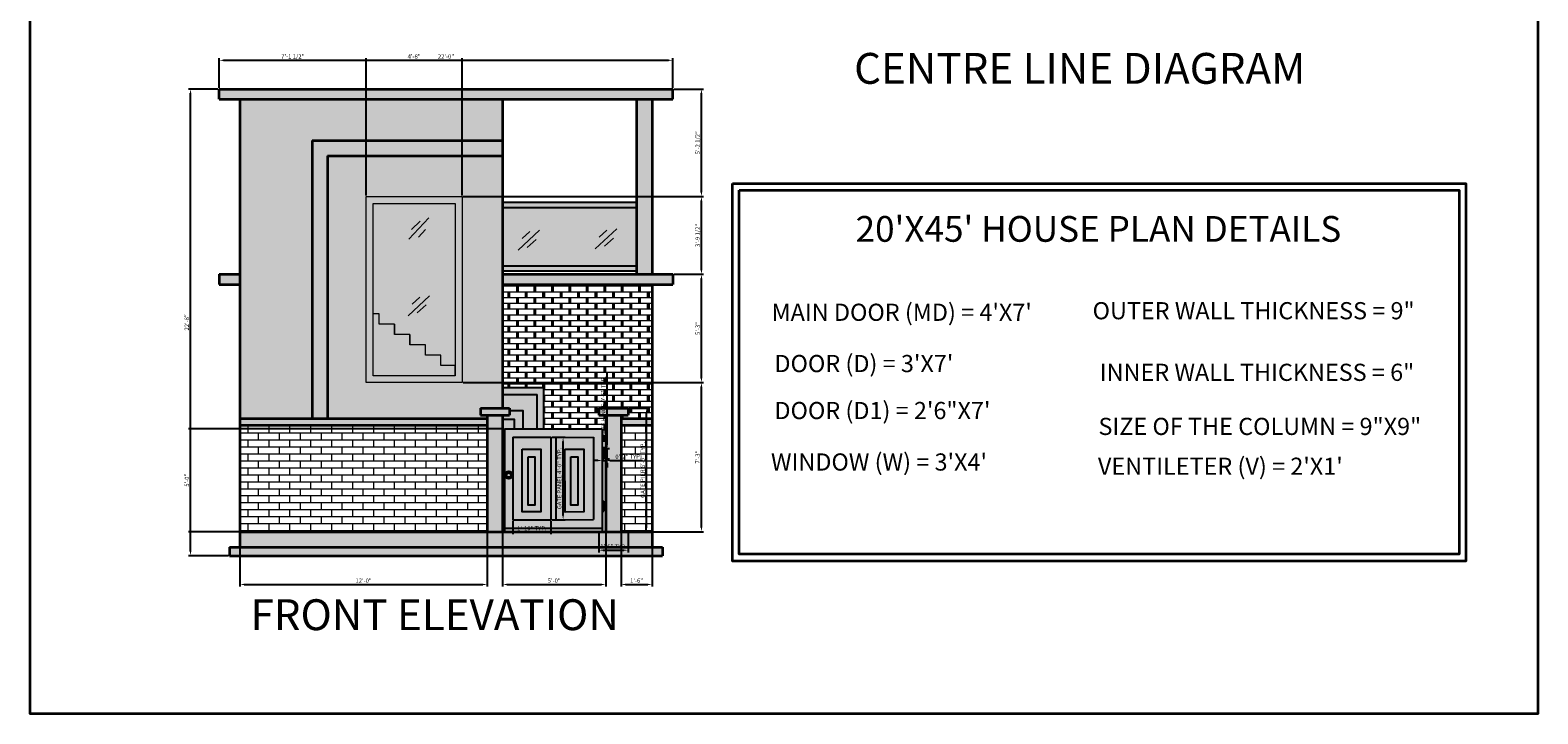
# Model space of a CAD drawing. Units: inches. Extents: x 2150 to 10686, y 1035 to 5077.
# Tile 10 of 12: x 9808 to 10686, y 1035 to 1433. Entities that reach past the tile are written whole.
import ezdxf

# ---------------------------------------------------------------- set-up
doc = ezdxf.new("R2010")
doc.units = ezdxf.units.IN
for name, color, linetype, lineweight in [('A-ANNO-DIMS', 2, 'Continuous', 18), ('A-ANNO-TEXT', 2, 'Continuous', 18), ('A-ANNO-TITL', 3, 'Continuous', 35), ('A-ANNO-TTLB', 7, 'Continuous', 35), ('A-ELEV', 7, 'Continuous', 35), ('A-ELEV-BASE-PATT', 251, 'Continuous', 13), ('A-ELEV-DOOR', 7, 'Continuous', 25), ('A-ELEV-DOOR-PATT', 17, 'Continuous', 13), ('A-ELEV-GLAZ', 7, 'Continuous', 18), ('A-ELEV-MASN-PATT', 32, 'Continuous', 13), ('A-ELEV-METL-PATT', 252, 'Continuous', 13), ('A-ELEV-RAIL', 7, 'Continuous', 25), ('A-ELEV-STRS', 7, 'Continuous', 18)]:
    doc.layers.add(name, color=color, linetype=linetype, lineweight=lineweight)
for name, color, linetype, lineweight, true_color in [('A-ELEV-CONC-PATT', 253, 'Continuous', 13, 0xb2a88f), ('A-ELEV-GLAZ-PATT', 141, 'Continuous', 13, 0xadddf7), ('A-ELEV-PATT', 253, 'Continuous', 13, 0xa5adc8), ('A-ELEV-TRIM-PATT', 85, 'Continuous', 13, 0x58ba48)]:
    doc.layers.add(name, color=color, linetype=linetype, lineweight=lineweight, true_color=true_color)
doc.styles.get("Standard").update_dxf_attribs({"font": 'arial.ttf'})
doc.dimstyles.new('ISO-25', dxfattribs={"dimtxt": 2.5, "dimasz": 2.5, "dimexe": 1.25, "dimexo": 0.625, "dimtad": 1, "dimdec": 0, "dimlunit": 3, "dimtxsty": 'Standard', "dimcen": 2.5, "dimadec": 0, "dimazin": 0, "dimtfac": 1, "dimtdec": 0, "dimtmove": 0, "dimatfit": 3, "dimfxl": 1, "dimarcsym": 0})

# ---------------------------------------------------------------- blocks, each defined once
blk = doc.blocks.new('GLASS-REFLECTION-COMPACT')
for p, q in [((0, 0), (11.74, 12.37)), ((1.57, 5.5), (6.55, 10.47)), ((5.63, 1.12), (9.83, 5.5))]:
    blk.add_line(p, q)
blk = doc.blocks.new('GATE-PIER-CAPPED')
for p, q in [((0, 72), (0, 68)), ((0, 72), (17, 72)), ((17, 72), (17, 68)), ((0, 68), (17, 68)), ((4, 68), (4, 0)), ((13, 68), (13, 0))]:
    blk.add_line(p, q)
blk = doc.blocks.new('GATE-INSET-PANEL-22')
for p, q in [((0, 48), (0, 0)), ((0, 48), (22, 48)), ((22, 48), (22, 0)), ((0, 0), (22, 0))]:
    blk.add_line(p, q)
for points in [[(5.38, 41.12), (16.31, 41.12), (16.31, 4.48), (5.38, 4.48)], [(8.77, 36.65), (12.8, 36.65), (12.8, 8.4), (8.77, 8.4)]]:
    blk.add_lwpolyline(points, close=True)
blk = doc.blocks.new('GATE-HINGE-6IN')
for p, q in [((0, 6), (1, 6)), ((0, 0), (1, 0)), ((1, 6), (1, 0)), ((1, 4), (2, 4)), ((1, 2), (2, 2))]:
    blk.add_line(p, q)
blk = doc.blocks.new('*D68')
at = {"layer": 'A-ANNO-DIMS', "color": 0, "lineweight": -2, "transparency": 16777216}
for p, q in [((10157.13, 1213.1), (10168.56, 1213.1)), ((10167.31, 1143.6), (10167.31, 1210.6)), ((10157.13, 1141.1), (10168.56, 1141.1))]:
    blk.add_line(p, q, dxfattribs=at)
at = {"layer": 'A-ANNO-DIMS', "color": 0, "transparency": 16777216}
for points in [[(10166.89, 1210.6), (10167.72, 1210.6), (10167.31, 1213.1)], [(10166.89, 1143.6), (10167.72, 1143.6), (10167.31, 1141.1)]]:
    blk.add_solid(points, dxfattribs=at)
at = {"layer": 'Defpoints', "color": 0, "transparency": 16777216}
for p in [(10156.51, 1213.1), (10167.31, 1213.1), (10156.51, 1141.1)]:
    blk.add_point(p, dxfattribs=at)
at = {"layer": 'A-ANNO-DIMS', "color": 0, "transparency": 16777216, "insert": (10165.39, 1177.1), "char_height": 2.5, "attachment_point": 5, "rotation": 90}
blk.add_mtext('GATE PIER 6\'-0" TYP.', dxfattribs=at)
blk = doc.blocks.new('*D69')
at = {"layer": 'A-ANNO-DIMS', "color": 0, "lineweight": -2, "transparency": 16777216}
for p, q in [((10139.51, 1140.47), (10139.51, 1129.05)), ((10156.51, 1140.47), (10156.51, 1129.05)), ((10142.01, 1130.3), (10154.01, 1130.3))]:
    blk.add_line(p, q, dxfattribs=at)
at = {"layer": 'A-ANNO-DIMS', "color": 0, "transparency": 16777216}
for points in [[(10142.01, 1130.71), (10142.01, 1129.88), (10139.51, 1130.3)], [(10154.01, 1130.71), (10154.01, 1129.88), (10156.51, 1130.3)]]:
    blk.add_solid(points, dxfattribs=at)
at = {"layer": 'Defpoints', "color": 0, "transparency": 16777216}
for p in [(10139.51, 1141.1), (10156.51, 1141.1), (10156.51, 1130.3)]:
    blk.add_point(p, dxfattribs=at)
at = {"layer": 'A-ANNO-DIMS', "color": 0, "transparency": 16777216, "insert": (10148.01, 1132.2), "char_height": 2.5, "attachment_point": 5}
blk.add_mtext('1\'-5" TYP.', dxfattribs=at)
blk = doc.blocks.new('*D70')
at = {"layer": 'A-ANNO-DIMS', "color": 0, "lineweight": -2, "transparency": 16777216}
for p, q in [((10112.13, 1196.1), (10119.96, 1196.1)), ((10118.71, 1150.6), (10118.71, 1193.6)), ((10112.13, 1148.1), (10119.96, 1148.1))]:
    blk.add_line(p, q, dxfattribs=at)
at = {"layer": 'A-ANNO-DIMS', "color": 0, "transparency": 16777216}
for points in [[(10118.29, 1193.6), (10119.12, 1193.6), (10118.71, 1196.1)], [(10118.29, 1150.6), (10119.12, 1150.6), (10118.71, 1148.1)]]:
    blk.add_solid(points, dxfattribs=at)
at = {"layer": 'Defpoints', "color": 0, "transparency": 16777216}
for p in [(10111.51, 1196.1), (10118.71, 1196.1), (10111.51, 1148.1)]:
    blk.add_point(p, dxfattribs=at)
at = {"layer": 'A-ANNO-DIMS', "color": 0, "transparency": 16777216, "insert": (10116.79, 1172.1), "char_height": 2.5, "attachment_point": 5, "rotation": 90}
blk.add_mtext('GATE PANEL 4\'-0" TYP.', dxfattribs=at)
blk = doc.blocks.new('*D71')
at = {"layer": 'A-ANNO-DIMS', "color": 0, "lineweight": -2, "transparency": 16777216}
for p, q in [((10089.51, 1147.47), (10089.51, 1139.65)), ((10111.51, 1147.47), (10111.51, 1139.65)), ((10092.01, 1140.9), (10109.01, 1140.9))]:
    blk.add_line(p, q, dxfattribs=at)
at = {"layer": 'A-ANNO-DIMS', "color": 0, "transparency": 16777216}
for points in [[(10092.01, 1141.31), (10092.01, 1140.48), (10089.51, 1140.9)], [(10109.01, 1141.31), (10109.01, 1140.48), (10111.51, 1140.9)]]:
    blk.add_solid(points, dxfattribs=at)
at = {"layer": 'Defpoints', "color": 0, "transparency": 16777216}
for p in [(10089.51, 1148.1), (10111.51, 1148.1), (10111.51, 1140.9)]:
    blk.add_point(p, dxfattribs=at)
at = {"layer": 'A-ANNO-DIMS', "color": 0, "transparency": 16777216, "insert": (10100.51, 1142.8), "char_height": 2.5, "attachment_point": 5}
blk.add_mtext('1\'-10" TYP.', dxfattribs=at)
blk = doc.blocks.new('*D74')
at = {"layer": 'A-ANNO-DIMS', "color": 0, "lineweight": -2, "transparency": 16777216}
for p, q in [((10144.41, 1191.99), (10144.41, 1233.45)), ((10144.13, 1189.49), (10145.66, 1189.49)), ((10144.41, 1183.49), (10144.41, 1189.49)), ((10144.13, 1183.49), (10145.66, 1183.49)), ((10144.41, 1180.99), (10144.41, 1178.49))]:
    blk.add_line(p, q, dxfattribs=at)
at = {"layer": 'A-ANNO-DIMS', "color": 0, "transparency": 16777216}
for points in [[(10143.99, 1191.99), (10144.82, 1191.99), (10144.41, 1189.49)], [(10143.99, 1180.99), (10144.82, 1180.99), (10144.41, 1183.49)]]:
    blk.add_solid(points, dxfattribs=at)
at = {"layer": 'Defpoints', "color": 0, "transparency": 16777216}
for p in [(10143.51, 1189.49), (10144.41, 1189.49), (10143.51, 1183.49)]:
    blk.add_point(p, dxfattribs=at)
at = {"layer": 'A-ANNO-DIMS', "color": 0, "transparency": 16777216, "insert": (10142.49, 1213.97), "char_height": 2.5, "attachment_point": 5, "rotation": 90}
blk.add_mtext('GATE HINGE 0\'-6" TYP.', dxfattribs=at)
blk = doc.blocks.new('*D75')
at = {"layer": 'A-ANNO-DIMS', "color": 0, "lineweight": -2, "transparency": 16777216}
for p, q in [((10139.01, 1182.59), (10136.51, 1182.59)), ((10141.51, 1182.86), (10141.51, 1181.34)), ((10141.51, 1182.59), (10143.51, 1182.59)), ((10143.51, 1182.86), (10143.51, 1181.34)), ((10146.01, 1182.59), (10165, 1182.59))]:
    blk.add_line(p, q, dxfattribs=at)
at = {"layer": 'A-ANNO-DIMS', "color": 0, "transparency": 16777216}
for points in [[(10139.01, 1183), (10139.01, 1182.17), (10141.51, 1182.59)], [(10146.01, 1183), (10146.01, 1182.17), (10143.51, 1182.59)]]:
    blk.add_solid(points, dxfattribs=at)
at = {"layer": 'Defpoints', "color": 0, "transparency": 16777216}
for p in [(10141.51, 1183.49), (10143.51, 1183.49), (10143.51, 1182.59)]:
    blk.add_point(p, dxfattribs=at)
at = {"layer": 'A-ANNO-DIMS', "color": 0, "transparency": 16777216, "insert": (10156.75, 1184.49), "char_height": 2.5, "attachment_point": 5}
blk.add_mtext('0\'-2" TYP.', dxfattribs=at)
blk = doc.blocks.new('*D114')
at = {"layer": 'A-ANNO-DIMS', "color": 0, "lineweight": -2, "transparency": 16777216}
for p, q in [((9918.51, 1399.72), (9918.51, 1417.1)), ((9921.01, 1415.85), (10180.01, 1415.85)), ((10182.51, 1399.72), (10182.51, 1417.1))]:
    blk.add_line(p, q, dxfattribs=at)
at = {"layer": 'A-ANNO-DIMS', "color": 0, "transparency": 16777216}
for points in [[(9921.01, 1416.26), (9921.01, 1415.43), (9918.51, 1415.85)], [(10180.01, 1416.26), (10180.01, 1415.43), (10182.51, 1415.85)]]:
    blk.add_solid(points, dxfattribs=at)
at = {"layer": 'Defpoints', "color": 0, "transparency": 16777216}
for p in [(10182.51, 1415.85), (9918.51, 1399.1), (10182.51, 1399.1)]:
    blk.add_point(p, dxfattribs=at)
at = {"layer": 'A-ANNO-DIMS', "color": 0, "transparency": 16777216, "insert": (10050.51, 1417.75), "char_height": 2.5, "attachment_point": 5}
blk.add_mtext('22\'-0"', dxfattribs=at)
blk = doc.blocks.new('*D115')
at = {"layer": 'A-ANNO-DIMS', "color": 0, "lineweight": -2, "transparency": 16777216}
for p, q in [((9917.88, 1399.1), (9900.51, 1399.1)), ((9901.76, 1129.6), (9901.76, 1396.6)), ((9923.88, 1127.1), (9900.51, 1127.1))]:
    blk.add_line(p, q, dxfattribs=at)
at = {"layer": 'A-ANNO-DIMS', "color": 0, "transparency": 16777216}
for points in [[(9901.34, 1396.6), (9902.17, 1396.6), (9901.76, 1399.1)], [(9901.34, 1129.6), (9902.17, 1129.6), (9901.76, 1127.1)]]:
    blk.add_solid(points, dxfattribs=at)
at = {"layer": 'Defpoints', "color": 0, "transparency": 16777216}
for p in [(9901.76, 1399.1), (9918.51, 1399.1), (9924.51, 1127.1)]:
    blk.add_point(p, dxfattribs=at)
at = {"layer": 'A-ANNO-DIMS', "color": 0, "transparency": 16777216, "insert": (9899.86, 1263.1), "char_height": 2.5, "attachment_point": 5, "rotation": 90}
blk.add_mtext('22\'-8"', dxfattribs=at)
blk = doc.blocks.new('*D116')
at = {"layer": 'A-ANNO-DIMS', "color": 0, "lineweight": -2, "transparency": 16777216}
for p, q in [((10060.52, 1228.01), (10200.51, 1228.01)), ((10199.26, 1143.6), (10199.26, 1225.51)), ((10171.13, 1141.1), (10200.51, 1141.1))]:
    blk.add_line(p, q, dxfattribs=at)
at = {"layer": 'A-ANNO-DIMS', "color": 0, "transparency": 16777216}
for points in [[(10198.84, 1225.51), (10199.67, 1225.51), (10199.26, 1228.01)], [(10198.84, 1143.6), (10199.67, 1143.6), (10199.26, 1141.1)]]:
    blk.add_solid(points, dxfattribs=at)
at = {"layer": 'Defpoints', "color": 0, "transparency": 16777216}
for p in [(10059.9, 1228.01), (10199.26, 1228.01), (10170.51, 1141.1)]:
    blk.add_point(p, dxfattribs=at)
at = {"layer": 'A-ANNO-DIMS', "color": 0, "transparency": 16777216, "insert": (10197.36, 1184.55), "char_height": 2.5, "attachment_point": 5, "rotation": 90}
blk.add_mtext('7\'-3"', dxfattribs=at)
blk = doc.blocks.new('*D117')
at = {"layer": 'A-ANNO-DIMS', "color": 0, "lineweight": -2, "transparency": 16777216}
for p, q in [((10183.13, 1291.1), (10200.51, 1291.1)), ((10199.26, 1230.51), (10199.26, 1288.6)), ((10060.52, 1228.01), (10200.51, 1228.01))]:
    blk.add_line(p, q, dxfattribs=at)
at = {"layer": 'A-ANNO-DIMS', "color": 0, "transparency": 16777216}
for points in [[(10198.84, 1288.6), (10199.67, 1288.6), (10199.26, 1291.1)], [(10198.84, 1230.51), (10199.67, 1230.51), (10199.26, 1228.01)]]:
    blk.add_solid(points, dxfattribs=at)
at = {"layer": 'Defpoints', "color": 0, "transparency": 16777216}
for p in [(10182.51, 1291.1), (10199.26, 1291.1), (10059.9, 1228.01)]:
    blk.add_point(p, dxfattribs=at)
at = {"layer": 'A-ANNO-DIMS', "color": 0, "transparency": 16777216, "insert": (10197.36, 1259.55), "char_height": 2.5, "attachment_point": 5, "rotation": 90}
blk.add_mtext('5\'-3"', dxfattribs=at)
blk = doc.blocks.new('*D118')
at = {"layer": 'A-ANNO-DIMS', "color": 0, "lineweight": -2, "transparency": 16777216}
for p, q in [((10060.52, 1336.48), (10200.51, 1336.48)), ((10199.26, 1293.6), (10199.26, 1333.98)), ((10183.13, 1291.1), (10200.51, 1291.1))]:
    blk.add_line(p, q, dxfattribs=at)
at = {"layer": 'A-ANNO-DIMS', "color": 0, "transparency": 16777216}
for points in [[(10198.84, 1333.98), (10199.67, 1333.98), (10199.26, 1336.48)], [(10198.84, 1293.6), (10199.67, 1293.6), (10199.26, 1291.1)]]:
    blk.add_solid(points, dxfattribs=at)
at = {"layer": 'Defpoints', "color": 0, "transparency": 16777216}
for p in [(10059.9, 1336.48), (10199.26, 1336.48), (10182.51, 1291.1)]:
    blk.add_point(p, dxfattribs=at)
at = {"layer": 'A-ANNO-DIMS', "color": 0, "transparency": 16777216, "insert": (10197.34, 1313.79), "char_height": 2.5, "attachment_point": 5, "rotation": 90}
blk.add_mtext('3\'-9 1/2"', dxfattribs=at)
blk = doc.blocks.new('*D119')
at = {"layer": 'A-ANNO-DIMS', "color": 0, "lineweight": -2, "transparency": 16777216}
for p, q in [((10183.13, 1399.1), (10200.51, 1399.1)), ((10199.26, 1338.98), (10199.26, 1396.6)), ((10060.52, 1336.48), (10200.51, 1336.48))]:
    blk.add_line(p, q, dxfattribs=at)
at = {"layer": 'A-ANNO-DIMS', "color": 0, "transparency": 16777216}
for points in [[(10198.84, 1396.6), (10199.67, 1396.6), (10199.26, 1399.1)], [(10198.84, 1338.98), (10199.67, 1338.98), (10199.26, 1336.48)]]:
    blk.add_solid(points, dxfattribs=at)
at = {"layer": 'Defpoints', "color": 0, "transparency": 16777216}
for p in [(10182.51, 1399.1), (10199.26, 1399.1), (10059.9, 1336.48)]:
    blk.add_point(p, dxfattribs=at)
at = {"layer": 'A-ANNO-DIMS', "color": 0, "transparency": 16777216, "insert": (10197.34, 1367.79), "char_height": 2.5, "attachment_point": 5, "rotation": 90}
blk.add_mtext('5\'-2 1/2"', dxfattribs=at)
blk = doc.blocks.new('*D120')
at = {"layer": 'A-ANNO-DIMS', "color": 0, "lineweight": -2, "transparency": 16777216}
for p, q in [((9918.51, 1399.72), (9918.51, 1417.1)), ((9921.01, 1415.85), (10001.53, 1415.85)), ((10004.03, 1337.11), (10004.03, 1417.1))]:
    blk.add_line(p, q, dxfattribs=at)
at = {"layer": 'A-ANNO-DIMS', "color": 0, "transparency": 16777216}
for points in [[(9921.01, 1416.26), (9921.01, 1415.43), (9918.51, 1415.85)], [(10001.53, 1416.26), (10001.53, 1415.43), (10004.03, 1415.85)]]:
    blk.add_solid(points, dxfattribs=at)
at = {"layer": 'Defpoints', "color": 0, "transparency": 16777216}
for p in [(10004.03, 1415.85), (9918.51, 1399.1), (10004.03, 1336.48)]:
    blk.add_point(p, dxfattribs=at)
at = {"layer": 'A-ANNO-DIMS', "color": 0, "transparency": 16777216, "insert": (9961.27, 1417.77), "char_height": 2.5, "attachment_point": 5}
blk.add_mtext('7\'-1 1/2"', dxfattribs=at)
blk = doc.blocks.new('*D121')
at = {"layer": 'A-ANNO-DIMS', "color": 0, "lineweight": -2, "transparency": 16777216}
for p, q in [((10004.03, 1337.11), (10004.03, 1417.1)), ((10006.53, 1415.85), (10057.4, 1415.85)), ((10059.9, 1337.11), (10059.9, 1417.1))]:
    blk.add_line(p, q, dxfattribs=at)
at = {"layer": 'A-ANNO-DIMS', "color": 0, "transparency": 16777216}
for points in [[(10006.53, 1416.26), (10006.53, 1415.43), (10004.03, 1415.85)], [(10057.4, 1416.26), (10057.4, 1415.43), (10059.9, 1415.85)]]:
    blk.add_solid(points, dxfattribs=at)
at = {"layer": 'Defpoints', "color": 0, "transparency": 16777216}
for p in [(10059.9, 1415.85), (10004.03, 1336.48), (10059.9, 1336.48)]:
    blk.add_point(p, dxfattribs=at)
at = {"layer": 'A-ANNO-DIMS', "color": 0, "transparency": 16777216, "insert": (10031.96, 1417.75), "char_height": 2.5, "attachment_point": 5}
blk.add_mtext('4\'-8"', dxfattribs=at)
blk = doc.blocks.new('*D122')
at = {"layer": 'A-ANNO-DIMS', "color": 0, "lineweight": -2, "transparency": 16777216}
for p, q in [((9930.51, 1140.47), (9930.51, 1109.1)), ((10074.51, 1140.47), (10074.51, 1109.1)), ((9933.01, 1110.35), (10072.01, 1110.35))]:
    blk.add_line(p, q, dxfattribs=at)
at = {"layer": 'A-ANNO-DIMS', "color": 0, "transparency": 16777216}
for points in [[(9933.01, 1110.76), (9933.01, 1109.93), (9930.51, 1110.35)], [(10072.01, 1110.76), (10072.01, 1109.93), (10074.51, 1110.35)]]:
    blk.add_solid(points, dxfattribs=at)
at = {"layer": 'Defpoints', "color": 0, "transparency": 16777216}
for p in [(9930.51, 1141.1), (10074.51, 1141.1), (10074.51, 1110.35)]:
    blk.add_point(p, dxfattribs=at)
at = {"layer": 'A-ANNO-DIMS', "color": 0, "transparency": 16777216, "insert": (10002.51, 1112.25), "char_height": 2.5, "attachment_point": 5}
blk.add_mtext('12\'-0"', dxfattribs=at)
blk = doc.blocks.new('*D123')
at = {"layer": 'A-ANNO-DIMS', "color": 0, "lineweight": -2, "transparency": 16777216}
for p, q in [((10152.51, 1140.47), (10152.51, 1109.1)), ((10170.51, 1140.47), (10170.51, 1109.1)), ((10155.01, 1110.35), (10168.01, 1110.35))]:
    blk.add_line(p, q, dxfattribs=at)
at = {"layer": 'A-ANNO-DIMS', "color": 0, "transparency": 16777216}
for points in [[(10155.01, 1110.76), (10155.01, 1109.93), (10152.51, 1110.35)], [(10168.01, 1110.76), (10168.01, 1109.93), (10170.51, 1110.35)]]:
    blk.add_solid(points, dxfattribs=at)
at = {"layer": 'Defpoints', "color": 0, "transparency": 16777216}
for p in [(10152.51, 1141.1), (10170.51, 1141.1), (10170.51, 1110.35)]:
    blk.add_point(p, dxfattribs=at)
at = {"layer": 'A-ANNO-DIMS', "color": 0, "transparency": 16777216, "insert": (10161.51, 1112.25), "char_height": 2.5, "attachment_point": 5}
blk.add_mtext('1\'-6"', dxfattribs=at)
blk = doc.blocks.new('*D124')
at = {"layer": 'A-ANNO-DIMS', "color": 0, "lineweight": -2, "transparency": 16777216}
for p, q in [((10083.51, 1140.47), (10083.51, 1109.1)), ((10143.51, 1140.47), (10143.51, 1109.1)), ((10086.01, 1110.35), (10141.01, 1110.35))]:
    blk.add_line(p, q, dxfattribs=at)
at = {"layer": 'A-ANNO-DIMS', "color": 0, "transparency": 16777216}
for points in [[(10086.01, 1110.76), (10086.01, 1109.93), (10083.51, 1110.35)], [(10141.01, 1110.76), (10141.01, 1109.93), (10143.51, 1110.35)]]:
    blk.add_solid(points, dxfattribs=at)
at = {"layer": 'Defpoints', "color": 0, "transparency": 16777216}
for p in [(10083.51, 1141.1), (10143.51, 1141.1), (10143.51, 1110.35)]:
    blk.add_point(p, dxfattribs=at)
at = {"layer": 'A-ANNO-DIMS', "color": 0, "transparency": 16777216, "insert": (10113.51, 1112.25), "char_height": 2.5, "attachment_point": 5}
blk.add_mtext('5\'-0"', dxfattribs=at)
blk = doc.blocks.new('*D125')
at = {"layer": 'A-ANNO-DIMS', "color": 0, "lineweight": -2, "transparency": 16777216}
for p, q in [((10083.88, 1201.1), (9900.51, 1201.1)), ((9901.76, 1143.6), (9901.76, 1198.6)), ((10083.88, 1141.1), (9900.51, 1141.1))]:
    blk.add_line(p, q, dxfattribs=at)
at = {"layer": 'A-ANNO-DIMS', "color": 0, "transparency": 16777216}
for points in [[(9901.34, 1198.6), (9902.17, 1198.6), (9901.76, 1201.1)], [(9901.34, 1143.6), (9902.17, 1143.6), (9901.76, 1141.1)]]:
    blk.add_solid(points, dxfattribs=at)
at = {"layer": 'Defpoints', "color": 0, "transparency": 16777216}
for p in [(9901.76, 1201.1), (10084.51, 1201.1), (10084.51, 1141.1)]:
    blk.add_point(p, dxfattribs=at)
at = {"layer": 'A-ANNO-DIMS', "color": 0, "transparency": 16777216, "insert": (9899.86, 1171.1), "char_height": 2.5, "attachment_point": 5, "rotation": 90}
blk.add_mtext('5\'-0"', dxfattribs=at)

msp = doc.modelspace()

# ---------------------------------------------------------------- hatches: boundary and pattern name
at = {"layer": 'A-ELEV-BASE-PATT'}
h = msp.add_hatch(color=256, dxfattribs=at)
h.dxf.hatch_style = 1
h.paths.add_polyline_path([(10170.51, 1132.1), (10170.51, 1141.1), (9930.51, 1141.1), (9930.51, 1132.1)])
h = msp.add_hatch(color=256, dxfattribs=at)
h.dxf.hatch_style = 1
h.paths.add_polyline_path([(10176.51, 1132.1), (9924.51, 1132.1), (9924.51, 1127.1), (10176.51, 1127.1)])
at = {"layer": 'A-ELEV-CONC-PATT'}
h = msp.add_hatch(dxfattribs=at)
h.set_pattern_fill('AR-CONC', color=256, scale=0.03)
h.set_pattern_definition([(50, (3083.3583, -475.9), (5.46554, -0.4781726), [0.5715, -6.2865]), (355, (3083.3583, -475.9), (-1.0573026, 5.7317054), [0.4572, -5.0292175]), (100.451445, (3083.814, -475.94), (4.4082374, 5.2535326), [0.4857003, -5.3427073]), (46.1842, (3083.358, -474.376), (8.132371, -1.26127), [0.85725, -9.42975]), (96.63556, (3084.036, -474.481), (7.122124, 7.422784), [0.728551, -8.014068]), (351.18415, (3083.358, -474.376), (7.122124, 7.422784), [0.685799, -7.543792]), (21, (3084.1203, -474.757), (4.5484317, -3.067956), [0.5715, -6.2865]), (326, (3084.1203, -474.757), (1.854061, 5.525639), [0.4572, -5.0292]), (71.451445, (3084.4994, -475.013), (6.4024926, 2.457683), [0.4857003, -5.342698]), (37.5, (3083.3583, -475.9001), (0.0926581, 2.53665117), [0, -4.96824, 0, -5.1054, 0, -5.04825]), (7.5, (3083.3583, -475.9), (2.0045899, 3.0054172), [0, -2.91084, 0, -4.85394, 0, -1.92405]), (327.5, (3081.659, -475.9001), (4.06771786, -0.1718623), [0, -1.905, 0, -5.9436, 0, -7.8867]), (317.5, (3080.897, -475.9), (4.4438754, 0.7627947), [0, -2.4765, 0, -3.94716, 0, -5.6007])])
h.paths.add_polyline_path([(9981.51, 1360.1), (10083.51, 1360.1), (10083.51, 1369.1), (9972.51, 1369.1), (9972.51, 1207.1), (9981.51, 1207.1)])
h.paths.add_polyline_path([(10083.51, 1291.1), (10083.51, 1285.1), (10182.51, 1285.1), (10182.51, 1291.1)])
h.paths.add_polyline_path([(9930.51, 1285.1), (9930.51, 1291.1), (9918.51, 1291.1), (9918.51, 1285.1)])
h.paths.add_polyline_path([(10182.51, 1393.1), (10182.51, 1399.1), (9918.51, 1399.1), (9918.51, 1393.1)])
at = {"layer": 'A-ELEV-DOOR-PATT'}
h = msp.add_hatch(color=256, dxfattribs=at)
h.dxf.hatch_style = 1
h.paths.add_polyline_path([(10103.51, 1221.1), (10103.51, 1201.1), (10107.51, 1201.1), (10107.51, 1225.1), (10083.51, 1225.1), (10083.51, 1221.1)])
h.paths.add_polyline_path([(10095.48, 1211.51), (10087.51, 1211.51), (10087.51, 1209.1), (10083.51, 1209.1), (10083.51, 1206.51), (10090.48, 1206.51), (10090.48, 1201.1), (10095.48, 1201.1)], flags=17)
h = msp.add_hatch(color=256, dxfattribs=at)
h.dxf.hatch_style = 1
h.paths.add_polyline_path([(10103.51, 1221.1), (10083.51, 1221.1), (10083.51, 1213.1), (10087.51, 1213.1), (10087.51, 1211.51), (10095.48, 1211.51), (10095.48, 1201.1), (10103.51, 1201.1)])
h.paths.add_polyline_path([(10090.48, 1206.51), (10083.51, 1206.51), (10083.51, 1141.1), (10084.51, 1141.1), (10084.51, 1201.1), (10090.48, 1201.1)])
h = msp.add_hatch(color=256, dxfattribs=at)
h.dxf.hatch_style = 1
h.paths.add_polyline_path([(10084.51, 1143.1), (10141.51, 1143.1), (10141.51, 1201.1), (10084.51, 1201.1)])
h.paths.add_polyline_path([(10089.51, 1196.1), (10111.51, 1196.1), (10111.51, 1148.1), (10089.51, 1148.1)], flags=16)
h.paths.add_polyline_path([(10094.89, 1189.22), (10105.82, 1189.22), (10105.82, 1152.58), (10094.89, 1152.58)], flags=0)
h.paths.add_polyline_path([(10098.28, 1184.75), (10102.31, 1184.75), (10102.31, 1156.49), (10098.28, 1156.49)], flags=0)
h.paths.add_polyline_path([(10114.51, 1196.1), (10136.51, 1196.1), (10136.51, 1148.1), (10114.51, 1148.1)], flags=16)
h.paths.add_polyline_path([(10119.85, 1189.22), (10130.78, 1189.22), (10130.78, 1152.58), (10119.85, 1152.58)], flags=0)
h.paths.add_polyline_path([(10123.09, 1184.75), (10127.13, 1184.75), (10127.13, 1156.49), (10123.09, 1156.49)], flags=0)
h.paths.add_polyline_path([(10094.89, 1152.58), (10105.82, 1152.58), (10105.82, 1189.22), (10094.89, 1189.22)], flags=0)
at = {"layer": 'A-ELEV-GLAZ-PATT'}
h = msp.add_hatch(color=256, dxfattribs=at)
h.dxf.hatch_style = 1
h.paths.add_polyline_path([(10055.9, 1332.48), (10008.03, 1332.48), (10008.03, 1268.01), (10011.51, 1268.01), (10011.51, 1262.01), (10020.51, 1262.01), (10020.51, 1256.01), (10029.51, 1256.01), (10029.51, 1250.01), (10038.51, 1250.01), (10038.51, 1244.01), (10047.51, 1244.01), (10047.51, 1238.01), (10055.9, 1238.01)])
h.paths.add_polyline_path([(10047.51, 1244.01), (10038.51, 1244.01), (10038.51, 1250.01), (10029.51, 1250.01), (10029.51, 1256.01), (10020.51, 1256.01), (10020.51, 1262.01), (10011.51, 1262.01), (10011.51, 1268.01), (10008.03, 1268.01), (10008.03, 1232.01), (10055.9, 1232.01), (10055.9, 1238.01), (10047.51, 1238.01)])
h = msp.add_hatch(color=256, dxfattribs=at)
h.dxf.hatch_style = 1
h.paths.add_polyline_path([(10083.51, 1330.1), (10083.51, 1296.1), (10161.51, 1296.1), (10161.51, 1330.1)])
at = {"layer": 'A-ELEV-MASN-PATT'}
h = msp.add_hatch(dxfattribs=at)
h.set_pattern_fill('GRAVEL', color=256, scale=0.4)
h.set_pattern_definition([(228.012788, (3090.6735, -465.7401), (-81.28000001, -91.439999994), [1.366886, -135.321935]), (184.969741, (3089.75913, -466.7561), (121.919999952, 10.16000058), [2.345619, -232.216196]), (132.510447, (3087.4223, -466.9593), (101.600000043, -111.75999996), [1.653926, -163.738891]), (267.273689, (3083.45993, -469.4993), (10.16000002, 203.2), [2.136018, -211.46575]), (292.833654, (3083.35833, -471.6329), (-50.800000004, 121.919999998), [2.094535, -207.359231]), (357.273689, (3084.17113, -473.5633), (-203.2, 10.16000002), [2.136018, -211.46575]), (37.6942405, (3086.30473, -473.6649), (-132.079999994, -101.600000008), [2.824775, -279.652461]), (72.2553284, (3088.53993, -471.9377), (71.12000002, 223.519999994), [2.666878, -264.021026]), (121.429566, (3089.35273, -469.3977), (-81.28000001, 132.079999993), [2.143252, -212.182183]), (175.236358, (3088.2351, -467.5689), (111.76, -10.16000002), [2.446853, -119.895748]), (222.397438, (3085.79673, -467.3657), (-121.919999996, -111.760000004), [3.164312, -313.26709]), (138.814075, (3093.5183, -469.6009), (-71.12, 60.96), [1.080018, -106.922263]), (171.4692344, (3092.70553, -468.8897), (132.080000004, -20.319999977), [2.054728, -203.418556]), (225, (3090.6735, -468.585), (-1e-15, -10.16), [1.436837, -12.931572]), (203.19859, (3089.9623, -467.3657), (50.8, 20.32), [0.773765, -76.60249]), (291.80141, (3089.2511, -467.6705), (-10.16, 30.48), [1.094262, -53.619012]), (30.963757, (3089.6575, -468.6865), (30.48, 20.32), [1.777279, -57.465193]), (161.56505, (3091.1815, -467.772), (20.32, -10.16), [1.285149, -30.843592]), (16.38954, (3083.35833, -467.6705), (101.6, 30.48), [1.800352, -178.235307]), (70.346176, (3085.0855, -467.1625), (-40.640000004, -111.76), [1.510396, -149.528863]), (293.19859, (3091.1815, -465.7401), (-20.32, 50.8), [1.54752, -75.828734]), (343.61046, (3091.79113, -467.1625), (-101.6, 30.479999993), [1.800352, -178.235307]), (339.443955, (3083.3583, -473.9697), (-50.8, 20.32), [1.736141, -85.070937]), (294.775141, (3084.9839, -474.5793), (-50.80000006, 111.75999997), [1.454688, -144.014374]), (66.80141, (3091.2831, -475.9001), (20.32, 50.8), [1.54752, -75.828734]), (17.354025, (3091.89273, -474.4777), (-132.079999997, -40.64000001), [1.703131, -168.609504]), (69.443955, (3086.3047, -475.9001), (-20.32, -50.8), [0.86807, -85.939008]), (101.309932, (3090.6735, -475.9001), (-10.16, 40.64), [0.518058, -51.28798]), (165.963757, (3090.572, -475.392), (30.48, -10.16), [2.094535, -39.796218]), (186.009006, (3088.53993, -474.8841), (101.6, 10.160000005), [1.941068, -192.16546]), (303.690068, (3089.6575, -469.601), (-10.16, 20.32), [1.465296, -35.167105]), (353.1572266, (3090.47033, -470.8201), (172.72, -20.31999999), [2.558227, -253.264036]), (60.945396, (3093.0103, -471.1249), (-40.64, -71.12), [1.046033, -103.557569]), (90, (3093.518, -470.211), (-10.16, 10.16), [0.6096, -9.5504]), (120.256437, (3088.3367, -474.5793), (40.639999995, -71.12), [1.411468, -139.735763]), (48.012787, (3087.6255, -473.3601), (81.28000001, 91.439999994), [2.733772, -133.955049]), (0, (3089.454, -471.328), (10.16, 10.16), [2.6416, -7.5184]), (325.304846, (3092.0959, -471.3281), (101.60000004, -71.119999945), [1.606438, -159.037267]), (254.054604, (3093.4167, -472.2425), (-10.16, -40.64), [1.479316, -72.4866]), (207.6459754, (3093.01033, -473.6649), (-193.040000007, -101.599999987), [2.40858, -238.449858]), (175.426079, (3090.87673, -474.7825), (-132.08, 10.16), [2.548118, -252.263386])])
h.paths.add_polyline_path([(9972.51, 1369.1), (10083.51, 1369.1), (10083.51, 1393.1), (9930.51, 1393.1), (9930.51, 1207.1), (9972.51, 1207.1)])
h = msp.add_hatch(dxfattribs=at)
h.set_pattern_fill('BRSTONE', color=256, scale=0.4)
h.set_pattern_definition([(0, (3083.3583, -475.9), (0, 3.3528), []), (90, (3092.5023, -475.9), (-5.08, 3.3528), [3.3528, -3.3528]), (90, (3091.4863, -475.9), (-5.08, 3.3528), [3.3528, -3.3528]), (0, (3092.5023, -475.3413), (5.08, 3.3528), [-9.144, 1.016]), (0, (3092.5023, -474.7825), (5.08, 3.3528), [-9.144, 1.016]), (0, (3092.5023, -474.2237), (5.08, 3.3528), [-9.144, 1.016]), (0, (3092.5023, -473.665), (5.08, 3.3528), [-9.144, 1.016]), (0, (3092.5023, -473.106), (5.08, 3.3528), [-9.144, 1.016])])
h.paths.add_polyline_path([(10170.51, 1285.1), (10083.51, 1285.1), (10083.51, 1225.1), (10107.51, 1225.1), (10107.51, 1201.1), (10141.51, 1201.1), (10141.51, 1189.49), (10142.51, 1189.49), (10142.51, 1187.49), (10143.51, 1187.49), (10143.51, 1209.1), (10139.51, 1209.1), (10139.51, 1213.1), (10156.51, 1213.1), (10156.51, 1209.1), (10152.51, 1209.1), (10152.51, 1207.1), (10170.51, 1207.1)])
h = msp.add_hatch(dxfattribs=at)
h.set_pattern_fill('AR-BRSTD', color=256, scale=0.06)
h.set_pattern_definition([(0, (3083.3583, -475.9), (0, 4.064508), []), (90, (3083.3583, -475.9), (-6.096, 4.064508), [4.064508, -4.064508])])
h.paths.add_polyline_path([(10074.51, 1141.1), (10074.51, 1203.1), (9930.51, 1203.1), (9930.51, 1141.1)])
h.paths.add_polyline_path([(10170.51, 1203.1), (10152.51, 1203.1), (10152.51, 1141.1), (10170.51, 1141.1)])
at = {"layer": 'A-ELEV-METL-PATT'}
h = msp.add_hatch(color=256, dxfattribs=at)
h.dxf.hatch_style = 1
h.paths.add_polyline_path([(10004.03, 1228.01), (10059.9, 1228.01), (10059.9, 1336.48), (10004.03, 1336.48)])
h.paths.add_polyline_path([(10008.03, 1232.01), (10055.9, 1232.01), (10055.9, 1332.48), (10008.03, 1332.48)], flags=16)
h = msp.add_hatch(color=256, dxfattribs=at)
h.dxf.hatch_style = 1
h.paths.add_polyline_path([(10161.51, 1330.1), (10161.51, 1333.1), (10083.51, 1333.1), (10083.51, 1330.1)])
h.paths.add_polyline_path([(10161.51, 1293.1), (10161.51, 1296.1), (10083.51, 1296.1), (10083.51, 1293.1)])
h = msp.add_hatch(color=256, dxfattribs=at)
h.dxf.hatch_style = 1
h.paths.add_polyline_path([(10111.51, 1196.1), (10089.51, 1196.1), (10089.51, 1148.1), (10111.51, 1148.1)])
h.paths.add_polyline_path([(10105.82, 1189.22), (10105.82, 1152.58), (10094.89, 1152.58), (10094.89, 1189.22)], flags=16)
h.paths.add_polyline_path([(10102.31, 1184.75), (10102.31, 1156.49), (10098.28, 1156.49), (10098.28, 1184.75)], flags=0)
h.paths.add_polyline_path([(10114.51, 1196.1), (10114.51, 1148.1), (10136.51, 1148.1), (10136.51, 1196.1)])
h.paths.add_polyline_path([(10119.85, 1189.22), (10130.78, 1189.22), (10130.78, 1152.58), (10119.85, 1152.58)], flags=16)
h.paths.add_polyline_path([(10123.09, 1184.75), (10127.13, 1184.75), (10127.13, 1156.49), (10123.09, 1156.49)], flags=0)
h = msp.add_hatch(color=256, dxfattribs=at)
h.dxf.hatch_style = 1
h.paths.add_polyline_path([(10143.51, 1185.49), (10142.51, 1185.49), (10142.51, 1183.49), (10141.51, 1183.49), (10141.51, 1158.97), (10142.51, 1158.97), (10142.51, 1156.97), (10143.51, 1156.97)])
h.paths.add_polyline_path([(10143.51, 1154.97), (10142.51, 1154.97), (10142.51, 1152.97), (10141.51, 1152.97), (10141.51, 1141.1), (10143.51, 1141.1)])
h.paths.add_polyline_path([(10141.51, 1143.1), (10084.51, 1143.1), (10084.51, 1141.1), (10141.51, 1141.1)])
h = msp.add_hatch(color=256, dxfattribs=at)
h.dxf.hatch_style = 1
h.paths.add_polyline_path([(10105.82, 1189.22), (10094.89, 1189.22), (10094.89, 1152.58), (10105.82, 1152.58)])
h.paths.add_polyline_path([(10102.31, 1184.75), (10102.31, 1156.49), (10098.28, 1156.49), (10098.28, 1184.75)], flags=16)
h.paths.add_polyline_path([(10130.78, 1189.22), (10119.85, 1189.22), (10119.85, 1152.58), (10130.78, 1152.58)])
h.paths.add_polyline_path([(10127.13, 1184.75), (10127.13, 1156.49), (10123.09, 1156.49), (10123.09, 1184.75)], flags=16)
h.paths.add_polyline_path([(10143.51, 1187.49), (10142.51, 1187.49), (10142.51, 1185.49), (10143.51, 1185.49)])
h.paths.add_polyline_path([(10142.51, 1189.49), (10141.51, 1189.49), (10141.51, 1183.49), (10142.51, 1183.49)])
h.paths.add_polyline_path([(10143.51, 1156.97), (10142.51, 1156.97), (10142.51, 1154.97), (10143.51, 1154.97)])
h.paths.add_polyline_path([(10142.51, 1158.97), (10141.51, 1158.97), (10141.51, 1152.97), (10142.51, 1152.97)])
h = msp.add_hatch(color=256, dxfattribs=at)
h.dxf.hatch_style = 1
h.paths.add_polyline_path([(10098.28, 1156.49), (10102.31, 1156.49), (10102.31, 1184.75), (10098.28, 1184.75)])
h.paths.add_polyline_path([(10127.13, 1184.75), (10123.09, 1184.75), (10123.09, 1156.49), (10127.13, 1156.49)])
at = {"layer": 'A-ELEV-PATT'}
h = msp.add_hatch(color=256, dxfattribs=at)
h.dxf.hatch_style = 1
h.paths.add_polyline_path([(10170.51, 1393.1), (10161.51, 1393.1), (10161.51, 1291.1), (10170.51, 1291.1)])
h.paths.add_polyline_path([(10083.51, 1209.1), (10074.51, 1209.1), (10074.51, 1141.1), (10083.51, 1141.1)])
h.paths.add_polyline_path([(10152.51, 1209.1), (10143.51, 1209.1), (10143.51, 1141.1), (10152.51, 1141.1)])
h = msp.add_hatch(color=256, dxfattribs=at)
h.dxf.hatch_style = 1
h.paths.add_polyline_path([(9981.51, 1360.1), (9981.51, 1207.1), (10074.51, 1207.1), (10074.51, 1209.1), (10070.51, 1209.1), (10070.51, 1213.1), (10083.51, 1213.1), (10083.51, 1360.1)])
h.paths.add_polyline_path([(10004.03, 1336.48), (10059.9, 1336.48), (10059.9, 1228.01), (10004.03, 1228.01)], flags=16)
h.paths.add_polyline_path([(10008.03, 1332.48), (10055.9, 1332.48), (10055.9, 1232.01), (10008.03, 1232.01)], flags=0)
at = {"layer": 'A-ELEV-TRIM-PATT'}
h = msp.add_hatch(color=256, dxfattribs=at)
h.dxf.hatch_style = 1
h.paths.add_polyline_path([(9930.51, 1207.1), (9930.51, 1203.1), (10074.51, 1203.1), (10074.51, 1207.1)])
h.paths.add_polyline_path([(10070.51, 1213.1), (10070.51, 1209.1), (10087.51, 1209.1), (10087.51, 1213.1)])
h.paths.add_polyline_path([(10139.51, 1213.1), (10139.51, 1209.1), (10156.51, 1209.1), (10156.51, 1213.1)])
h.paths.add_polyline_path([(10152.51, 1207.1), (10152.51, 1203.1), (10170.51, 1203.1), (10170.51, 1207.1)])

# ---------------------------------------------------------------- linework, layer by layer
at = {"layer": 'A-ANNO-TTLB'}
for points in [[(9808.35, 2090.85), (10686.34, 2090.85), (10686.34, 1034.91), (9808.35, 1034.91)], [(10217.27, 1344.08), (10644.43, 1344.08), (10644.43, 1123.96), (10217.27, 1123.96)], [(10221.27, 1340.08), (10640.43, 1340.08), (10640.43, 1127.96), (10221.27, 1127.96)]]:
    msp.add_lwpolyline(points, close=True, dxfattribs=at)
at = {"layer": 'A-ELEV'}
for p, q in [((9918.51, 1399.1), (10182.51, 1399.1)), ((9918.51, 1393.1), (9918.51, 1399.1)), ((10182.51, 1393.1), (10182.51, 1399.1)), ((9918.51, 1393.1), (10182.51, 1393.1)), ((9930.51, 1393.1), (9930.51, 1132.1)), ((10083.51, 1393.1), (10083.51, 1213.1)), ((10161.51, 1393.1), (10161.51, 1291.1)), ((10170.51, 1393.1), (10170.51, 1291.1)), ((9972.51, 1369.1), (9972.51, 1207.1)), ((9972.51, 1369.1), (10083.51, 1369.1)), ((9981.51, 1360.1), (9981.51, 1207.1)), ((9981.51, 1360.1), (10083.51, 1360.1)), ((9918.51, 1291.1), (9930.51, 1291.1)), ((9918.51, 1291.1), (9918.51, 1285.1)), ((10083.51, 1291.1), (10182.51, 1291.1)), ((10182.51, 1291.1), (10182.51, 1285.1)), ((9918.51, 1285.1), (9930.51, 1285.1)), ((10083.51, 1285.1), (10182.51, 1285.1)), ((10170.51, 1285.1), (10170.51, 1132.1)), ((9930.51, 1207.1), (10074.51, 1207.1)), ((9930.51, 1203.1), (10074.51, 1203.1)), ((10152.51, 1207.1), (10170.51, 1207.1)), ((10152.51, 1203.1), (10170.51, 1203.1)), ((9930.51, 1141.1), (10170.51, 1141.1)), ((9924.51, 1132.1), (10176.51, 1132.1)), ((9924.51, 1132.1), (9924.51, 1127.1)), ((9924.51, 1127.1), (10176.51, 1127.1)), ((10176.51, 1132.1), (10176.51, 1127.1))]:
    msp.add_line(p, q, dxfattribs=at)
at = {"layer": 'A-ELEV-DOOR'}
for p, q in [((10083.51, 1225.1), (10107.51, 1225.1)), ((10083.51, 1221.1), (10103.51, 1221.1)), ((10103.51, 1201.1), (10103.51, 1221.1)), ((10107.51, 1201.1), (10107.51, 1225.1)), ((10084.51, 1201.1), (10141.51, 1201.1)), ((10084.51, 1201.1), (10084.51, 1141.1)), ((10141.51, 1201.1), (10141.51, 1141.1)), ((10084.51, 1143.1), (10141.51, 1143.1))]:
    msp.add_line(p, q, dxfattribs=at)
for points in [[(10090.48, 1201.1), (10090.48, 1206.51), (10083.51, 1206.51)], [(10095.48, 1201.1), (10095.48, 1211.51), (10087.51, 1211.51)]]:
    msp.add_lwpolyline(points, dxfattribs=at)
for radius in [2.27, 1.27]:
    msp.add_circle((10087.02, 1174.1), radius, dxfattribs=at)
at = {"layer": 'A-ELEV-GLAZ'}
for points in [[(10004.03, 1336.48), (10059.9, 1336.48), (10059.9, 1228.01), (10004.03, 1228.01)], [(10008.03, 1332.48), (10055.9, 1332.48), (10055.9, 1232.01), (10008.03, 1232.01)]]:
    msp.add_lwpolyline(points, close=True, dxfattribs=at)
at = {"layer": 'A-ELEV-RAIL'}
for p, q in [((10083.51, 1333.1), (10161.51, 1333.1)), ((10083.51, 1330.1), (10161.51, 1330.1)), ((10083.51, 1296.1), (10161.51, 1296.1)), ((10083.51, 1293.1), (10161.51, 1293.1))]:
    msp.add_line(p, q, dxfattribs=at)
at = {"layer": 'A-ELEV-STRS'}
for p, q in [((10011.51, 1268.01), (10008.03, 1268.01)), ((10011.51, 1262.01), (10011.51, 1268.01)), ((10020.51, 1262.01), (10011.51, 1262.01)), ((10020.51, 1262.01), (10020.51, 1256.01)), ((10020.51, 1256.01), (10020.51, 1262.01)), ((10029.51, 1256.01), (10020.51, 1256.01)), ((10029.51, 1256.01), (10029.51, 1250.01)), ((10029.51, 1250.01), (10029.51, 1256.01)), ((10038.51, 1250.01), (10029.51, 1250.01)), ((10038.51, 1244.01), (10038.51, 1250.01)), ((10047.51, 1244.01), (10038.51, 1244.01)), ((10047.51, 1238.01), (10047.51, 1244.01)), ((10055.9, 1238.01), (10047.51, 1238.01)), ((10055.9, 1232.01), (10055.9, 1238.01))]:
    msp.add_line(p, q, dxfattribs=at)

# ---------------------------------------------------------------- block references
at = {"layer": 'A-ELEV'}
for p in [(10070.51, 1141.1), (10139.51, 1141.1)]:
    msp.add_blockref('GATE-PIER-CAPPED', p, dxfattribs=at)
at = {"layer": 'A-ELEV-DOOR'}
for name, p in [('GATE-INSET-PANEL-22', (10089.51, 1148.1)), ('GATE-HINGE-6IN', (10141.51, 1183.49)), ('GATE-HINGE-6IN', (10141.51, 1152.97))]:
    msp.add_blockref(name, p, dxfattribs=at)
at = {"layer": 'A-ELEV-DOOR', "rotation": 0.1203022421829881}
msp.add_blockref('GATE-INSET-PANEL-22', (10114.5, 1148.08), dxfattribs=at)
at = {"layer": 'A-ELEV-GLAZ'}
msp.add_blockref('GLASS-REFLECTION-COMPACT', (10028.84, 1311.66), dxfattribs=at)
for p, rotation in [((10104.97, 1316.8), 176.5128684824566), ((10149.9, 1317.57), 176.5128684824566), ((10040.94, 1278.63), 176.5128684824589)]:
    msp.add_blockref('GLASS-REFLECTION-COMPACT', p, dxfattribs=dict(at, rotation=rotation))

# ---------------------------------------------------------------- texts
at = {"layer": 'A-ANNO-TEXT', "char_height": 10, "attachment_point": 1}
for s, width, insert in [("MAIN DOOR (MD) = 4'X7'", 534.3022, (10240.12, 1273.98)), ('OUTER WALL THICKNESS = 9"', 563.4898, (10427.06, 1274.9)), ("DOOR (D) = 3'X7'", 493.5855, (10241.78, 1244.1)), ('INNER WALL THICKNESS = 6"', 484.0661, (10431.24, 1238.99)), ('DOOR (D1) = 2\'6"X7\'', 568.3712, (10241.78, 1216.71)), ('SIZE OF THE COLUMN = 9"X9"', 299.797, (10430.47, 1207.46)), ("WINDOW (W) = 3'X4'", 367.0146, (10239.75, 1186.72)), ("VENTILETER (V) = 2'X1'", 495.9273, (10430.16, 1184.24))]:
    msp.add_mtext_dynamic_manual_height_columns(s, width=width, gutter_width=12.5, heights=[0], dxfattribs=dict(at, insert=insert))
at = {"layer": 'A-ANNO-TITL', "attachment_point": 1}
for s, width, insert, char_height in [('CENTRE LINE DIAGRAM', 1010.6338, (10288.18, 1420.14), 18), ("20'X45' HOUSE PLAN DETAILS", 581.6987, (10289.03, 1325.08), 15), ('FRONT ELEVATION', 504.5501, (9936.65, 1101.7), 18)]:
    msp.add_mtext_dynamic_manual_height_columns(s, width=width, gutter_width=12.5, heights=[0], dxfattribs=dict(at, insert=insert, char_height=char_height))

# ---------------------------------------------------------------- dimensions: what is measured, and where the dimension line sits
at = {"layer": 'A-ANNO-DIMS'}
for base, p1, p2, picture, middle in [((10004.03, 1415.85), (9918.51, 1399.1), (10004.03, 1336.48), '*D120', (9961.27, 1417.77)), ((10182.51, 1415.85), (9918.51, 1399.1), (10182.51, 1399.1), '*D114', (10050.51, 1417.75)), ((10059.9, 1415.85), (10004.03, 1336.48), (10059.9, 1336.48), '*D121', (10031.96, 1417.75)), ((10074.51, 1110.35), (9930.51, 1141.1), (10074.51, 1141.1), '*D122', (10002.51, 1112.25)), ((10143.51, 1110.35), (10083.51, 1141.1), (10143.51, 1141.1), '*D124', (10113.51, 1112.25)), ((10170.51, 1110.35), (10152.51, 1141.1), (10170.51, 1141.1), '*D123', (10161.51, 1112.25))]:
    dim = msp.add_linear_dim(base=base, p1=p1, p2=p2, dimstyle='ISO-25', override={"dimdec": 1, "dimlfac": 1, "dimrnd": 0, "dimzin": 1, "dimdsep": 46, "dimlunit": 4, "dimfrac": 2}, dxfattribs=at)
    dim.commit()
    dim.dimension.update_dxf_attribs({"geometry": picture, "text_midpoint": middle})
for base, p1, p2, picture, middle in [((9901.76, 1399.1), (9924.51, 1127.1), (9918.51, 1399.1), '*D115', (9899.86, 1263.1)), ((10199.26, 1399.1), (10059.9, 1336.48), (10182.51, 1399.1), '*D119', (10197.34, 1367.79)), ((10199.26, 1336.48), (10182.51, 1291.1), (10059.9, 1336.48), '*D118', (10197.34, 1313.79)), ((10199.26, 1291.1), (10059.9, 1228.01), (10182.51, 1291.1), '*D117', (10197.36, 1259.55)), ((10199.26, 1228.01), (10170.51, 1141.1), (10059.9, 1228.01), '*D116', (10197.36, 1184.55)), ((9901.76, 1201.1), (10084.51, 1141.1), (10084.51, 1201.1), '*D125', (9899.86, 1171.1))]:
    dim = msp.add_linear_dim(base=base, p1=p1, p2=p2, angle=90, dimstyle='ISO-25', override={"dimdec": 1, "dimlfac": 1, "dimrnd": 0, "dimzin": 1, "dimdsep": 46, "dimlunit": 4, "dimfrac": 2}, dxfattribs=at)
    dim.commit()
    dim.dimension.update_dxf_attribs({"geometry": picture, "text_midpoint": middle})
for base, p1, p2, text, picture, middle in [((10144.41, 1189.49), (10143.51, 1183.49), (10143.51, 1189.49), 'GATE HINGE <> TYP.', '*D74', (10142.49, 1213.97)), ((10167.31, 1213.1), (10156.51, 1141.1), (10156.51, 1213.1), 'GATE PIER <> TYP.', '*D68', (10165.39, 1177.1)), ((10118.71, 1196.1), (10111.51, 1148.1), (10111.51, 1196.1), 'GATE PANEL <> TYP.', '*D70', (10116.79, 1172.1))]:
    dim = msp.add_linear_dim(base=base, p1=p1, p2=p2, angle=90, text=text, dimstyle='ISO-25', override={"dimdec": 1, "dimlfac": 1, "dimrnd": 0, "dimzin": 1, "dimdsep": 46, "dimlunit": 4, "dimfrac": 2}, dxfattribs=at)
    dim.commit()
    dim.dimension.update_dxf_attribs({"geometry": picture, "text_midpoint": middle})
for base, p1, p2, picture, middle in [((10143.51, 1182.59), (10141.51, 1183.49), (10143.51, 1183.49), '*D75', (10156.75, 1184.49)), ((10111.51, 1140.9), (10089.51, 1148.1), (10111.51, 1148.1), '*D71', (10100.51, 1142.8)), ((10156.51, 1130.3), (10139.51, 1141.1), (10156.51, 1141.1), '*D69', (10148.01, 1132.2))]:
    dim = msp.add_linear_dim(base=base, p1=p1, p2=p2, text='<> TYP.', dimstyle='ISO-25', override={"dimdec": 1, "dimlfac": 1, "dimrnd": 0, "dimzin": 1, "dimdsep": 46, "dimlunit": 4, "dimfrac": 2}, dxfattribs=at)
    dim.commit()
    dim.dimension.update_dxf_attribs({"geometry": picture, "text_midpoint": middle})

doc.saveas('drawing.dxf')
